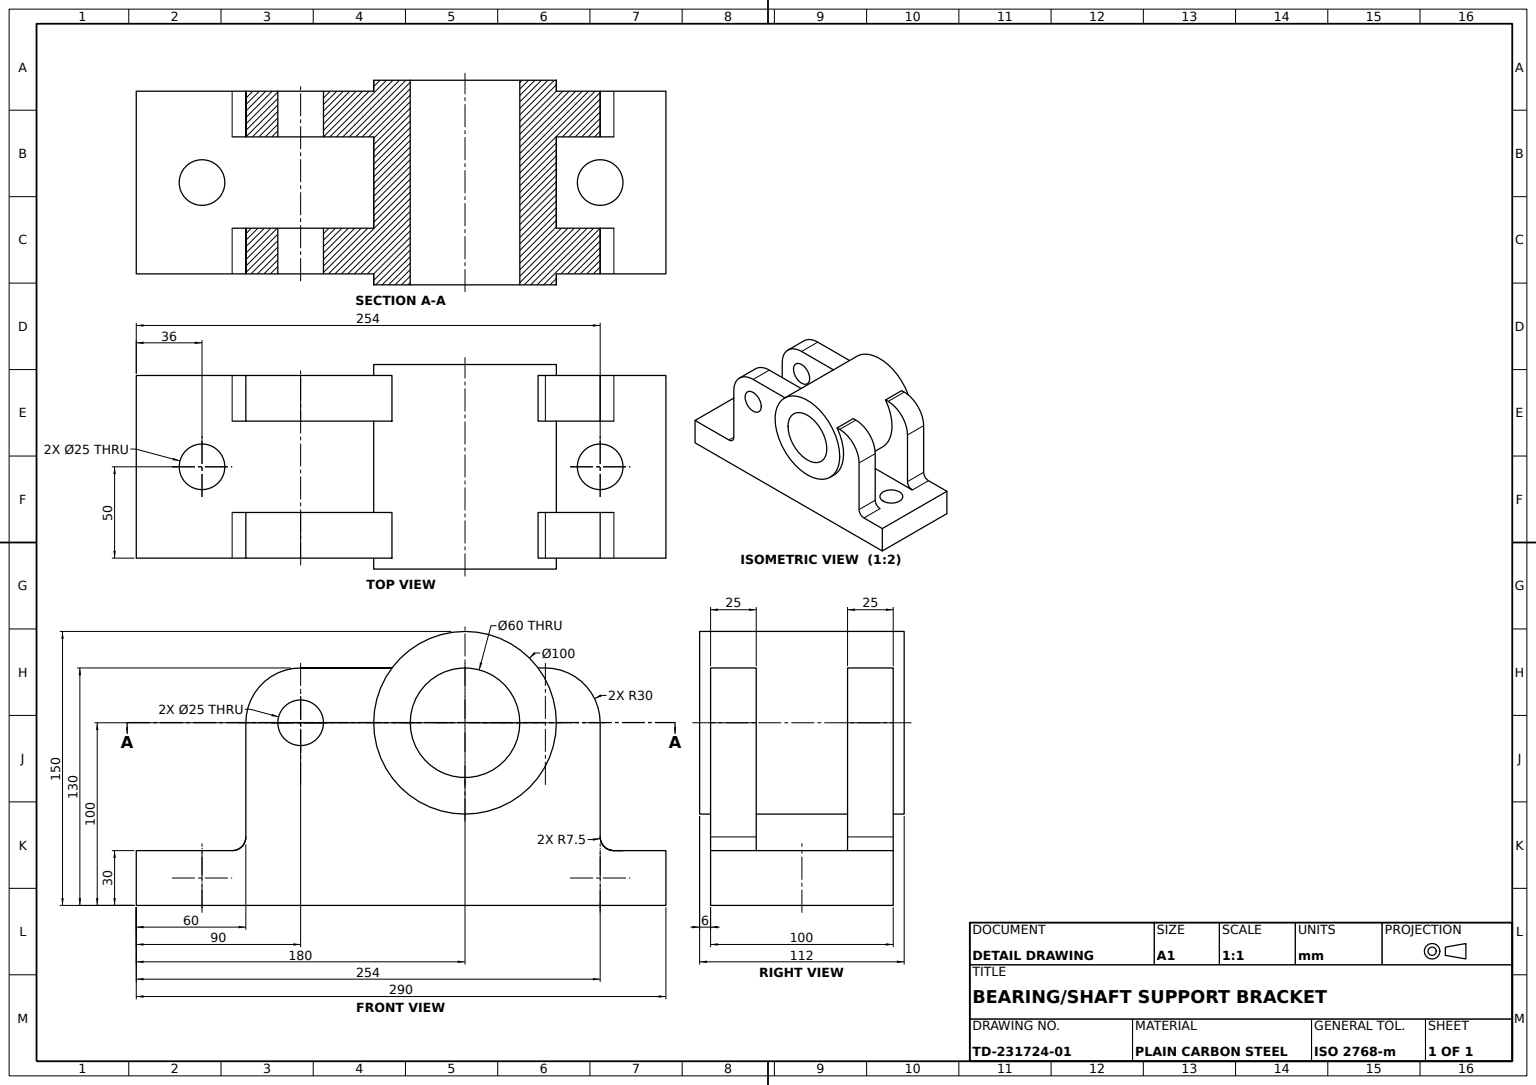
from build123d import *

# Parameters (mm, degrees)
BASE_PLATE_SKETCH_W         = 290
BASE_PLATE_SKETCH_H         = 30
BASE_PLATE_DEPTH            = 50
BEARING_BOSS_SKETCH_R       = 50
BEARING_BOSS_SKETCH_R_2     = 30
BEARING_BOSS_DEPTH          = 56
BASE_MOUNTING_CUT_SKETCH_R  = 12.5
BASE_MOUNTING_CUT_DEPTH     = 56
SUPPORT_LUG_SKETCH_W        = 194
SUPPORT_LUG_SKETCH_H        = 25
SUPPORT_LUG_DEPTH           = 130
LUG_PIN_HOLE_SKETCH_R       = 12.5
LUG_PIN_HOLE_25_DEPTH       = 65
LUG_PROFILE_CUT_DEPTH       = 130
HOUSING_CLEARANCE_CUT_DEPTH = 110
BEARING_START               = -120
BEARING_BORE_SKETCH_R       = 30
BEARING_BORE_60_DEPTH       = 120
RIB_1_DEPTH                 = 25
RIB_2_DEPTH                 = 25
RIB_3_DEPTH                 = 25
RIB_4_DEPTH                 = 25


with BuildPart() as part:
    # Base Plate Sketch → Base Plate (new, symmetric)
    with BuildSketch(Plane.XY):
        with Locations((-35, 15)):
            Rectangle(BASE_PLATE_SKETCH_W, BASE_PLATE_SKETCH_H)
    extrude(amount=BASE_PLATE_DEPTH, both=True)

    # Base Mounting Cut Sketch → Base Mounting Cut (cut, symmetric)
    with BuildSketch(Plane(origin=(0, 0, 0), x_dir=(1, 0, 0), z_dir=(0, 1, 0))):
        with Locations(Location((-144, 0, 0), (0, 0, 180))):
            Circle(BASE_MOUNTING_CUT_SKETCH_R)
        with Locations(Location((74, 0, 0), (0, 0, 180))):
            Circle(BASE_MOUNTING_CUT_SKETCH_R)
    extrude(amount=BASE_MOUNTING_CUT_DEPTH, both=True, mode=Mode.SUBTRACT)



with BuildPart() as body_2:
    # Bearing Boss Sketch → Bearing Boss (new, symmetric)
    with BuildSketch(Plane.XY):
        with Locations((0, 100)):
            Circle(BEARING_BOSS_SKETCH_R)
        with Locations((0, 100)):
            Circle(BEARING_BOSS_SKETCH_R_2, mode=Mode.SUBTRACT)
    extrude(amount=BEARING_BOSS_DEPTH, both=True)


with BuildPart() as part_1:
    add(part.part)

    add(body_2.part)  # Support Lug merges body 2
    # Support Lug Sketch → Support Lug (add)
    with BuildSketch(Plane(origin=(0, 0, 0), x_dir=(1, 0, 0), z_dir=(0, 1, 0))):
        with Locations((-23, -37.5)):
            Rectangle(SUPPORT_LUG_SKETCH_W, SUPPORT_LUG_SKETCH_H)
    support_lug = extrude(amount=SUPPORT_LUG_DEPTH)

    # Support Lug Mirror: Support Lug across plane
    add(support_lug.mirror(Plane.XY))

    # Lug Pin Hole Sketch → Lug Pin Hole Ø25 (cut, symmetric)
    with BuildSketch(Plane.XY):
        with Locations((-90, 100)):
            Circle(LUG_PIN_HOLE_SKETCH_R)
    extrude(amount=LUG_PIN_HOLE_25_DEPTH, both=True, mode=Mode.SUBTRACT)

    # Lug Profile Cut Sketch → Lug Profile Cut (cut)
    with BuildSketch(Plane.XY.offset(50)):
        with BuildLine():
            Line((-120, 100), (-120, 130))
            Line((-120, 130), (-90, 130))
            ThreePointArc((-90, 130), (-111.213203436, 121.213203436), (-120, 100))
        make_face()
    extrude(amount=-LUG_PROFILE_CUT_DEPTH, mode=Mode.SUBTRACT)

    # Housing Clearance Sketch → Housing Clearance Cut (cut)
    with BuildSketch(Plane.XY.offset(50)):
        with BuildLine():
            Line((74, 130), (44, 130))
            ThreePointArc((44, 130), (65.213203436, 121.213203436), (74, 100))
            Line((74, 100), (74, 130))
        make_face()
    extrude(amount=-HOUSING_CLEARANCE_CUT_DEPTH, mode=Mode.SUBTRACT)

    # Bearing Bore Sketch → Bearing Bore Ø60 (cut)
    with BuildSketch(Plane.XY.offset(56).offset(BEARING_START)):
        with Locations((0, 100)):
            Circle(BEARING_BORE_SKETCH_R)
    extrude(amount=BEARING_BORE_60_DEPTH, mode=Mode.SUBTRACT)

    # Rib 1 Sketch → Rib 1 (add)
    with BuildSketch(Plane.XY.offset(50)):
        with BuildLine():
            Line((-127.5, 30), (-120, 30))
            Line((-120, 30), (-120, 37.5))
            ThreePointArc((-120, 37.5), (-122.196699141, 32.196699141), (-127.5, 30))
        make_face()
    extrude(amount=-RIB_1_DEPTH)

    # Rib 2 Sketch → Rib 2 (add)
    with BuildSketch(Plane.XY.offset(-25)):
        with BuildLine():
            Line((-127.5, 30), (-120, 30))
            Line((-120, 30), (-120, 37.5))
            ThreePointArc((-120, 37.5), (-122.196699141, 32.196699141), (-127.5, 30))
        make_face()
    extrude(amount=-RIB_2_DEPTH)

    # Rib 3 Sketch → Rib 3 (add)
    with BuildSketch(Plane.XY.offset(50)):
        with BuildLine():
            Line((74, 37.5), (74, 30))
            Line((74, 30), (81.5, 30))
            ThreePointArc((81.5, 30), (76.196699141, 32.196699141), (74, 37.5))
        make_face()
    extrude(amount=-RIB_3_DEPTH)

    # Rib 4 Sketch → Rib 4 (add)
    with BuildSketch(Plane.XY.offset(-25)):
        with BuildLine():
            Line((74, 30), (81.5, 30))
            ThreePointArc((81.5, 30), (76.196699141, 32.196699141), (74, 37.5))
            Line((74, 37.5), (74, 30))
        make_face()
    extrude(amount=-RIB_4_DEPTH)


solid = part_1.part
